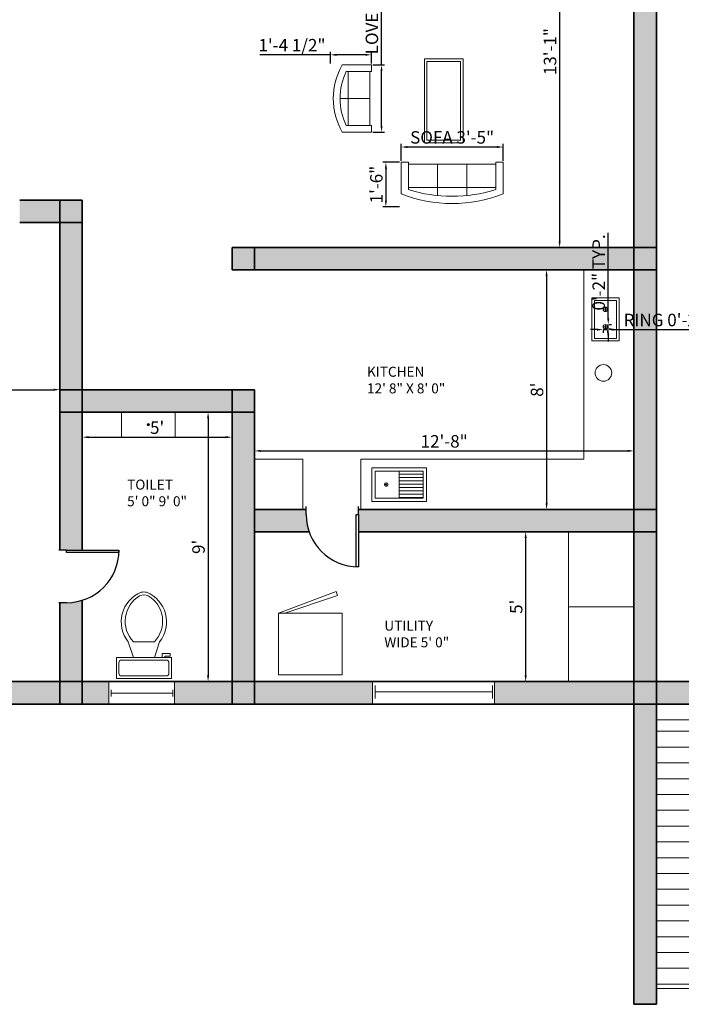
# Model space of a CAD drawing. Units: millimetres. Extents: x 2768 to 4359, y 795 to 1583.
# Tile 2 of 13: x 2961 to 3226, y 891 to 1286. Entities that reach past the tile are written whole.
import ezdxf

# ---------------------------------------------------------------- set-up
doc = ezdxf.new("R2010")
doc.units = ezdxf.units.MM
for name, color, linetype, lineweight in [('A-ANNO-DIMS', 90, 'Continuous', 18), ('A-AREA-IDEN', 190, 'Continuous', 18), ('A-DOOR-PATT', 251, 'Continuous', 13), ('A-EQPM', 50, 'Continuous', 18), ('A-FLOR-CASE', 50, 'Continuous', 18), ('A-FLOR-FIXT', 50, 'Continuous', 18), ('A-FLOR-FIXT-PATT', 50, 'Continuous', 13), ('A-WALL-PATT', 140, 'Continuous', 9), ('doors', 10, 'Continuous', 25), ('furniture', 50, 'Continuous', 18), ('iron shutter', 251, 'Continuous', 18), ('walls', 140, 'Continuous', 35), ('windows', 30, 'Continuous', 18)]:
    doc.layers.add(name, color=color, linetype=linetype, lineweight=lineweight)
doc.styles.get("Standard").update_dxf_attribs({"font": 'arial.ttf'})
doc.dimstyles.new('ISO-25', dxfattribs={"dimtxt": 5, "dimasz": 2.5, "dimexe": 1.25, "dimexo": 0.625, "dimtad": 1, "dimdec": 0, "dimlunit": 3, "dimtxsty": 'Standard', "dimcen": 2.5, "dimadec": 0, "dimazin": 0, "dimtfac": 1, "dimtdec": 0, "dimtmove": 0, "dimatfit": 3, "dimfxl": 1, "dimarcsym": 0})

# ---------------------------------------------------------------- blocks, each defined once
blk = doc.blocks.new('*U2')
for p, q in [((0, 0), (0, -6)), ((40, 0), (40, -6))]:
    blk.add_line(p, q)
blk.add_lwpolyline([(0, 0), (0, 40), (1.75, 40), (1.75, 0)], close=True)
blk.add_arc((0, 0), 40, 0, 90)
blk = doc.blocks.new('*U4')
for p, q in [((0, 4), (0, 0)), ((36, 4), (36, 0)), ((0, 2), (36, 2))]:
    blk.add_line(p, q)
blk = doc.blocks.new('*U5')
for p, q in [((0, 4), (0, 0)), ((0, 2), (36, 2)), ((36, 4), (36, 0))]:
    blk.add_line(p, q)
blk = doc.blocks.new('Toilet - top')
for p, q in [((9.5, -6), (9.5, -2)), ((-10, -8.5), (-8, -8.5)), ((-10, -9.5), (-10, -8.5)), ((-7, -9.5), (-10, -9.5)), ((-8, -8.5), (-8, -8)), ((-7, -8), (-7, -9.5)), ((-4, -8), (-6, -14)), ((4, -8), (6, -14)), ((4, -14), (-4, -14))]:
    blk.add_line(p, q)
blk.add_lwpolyline([(10.5, -8), (10.5, 0), (-10.5, 0), (-10.5, -8)], close=True)
for points in [[(-9.5, -2), (-9.5, -6)], [(8.5, -1), (-8.5, -1)], [(-8.5, -7), (8.5, -7)]]:
    blk.add_lwpolyline(points)
for centre, radius, start, end in [((-8.62, -1.88), 0.884, 81.8699, 188.1301), ((8.62, -1.88), 0.884, 351.8699, 98.1301), ((-8.62, -6.12), 0.884, 171.8699, 278.1301), ((8.62, -6.12), 0.884, 261.8699, 8.1301), ((3.52, -21.58), 12.17, 141.4691, 247.9714), ((4.2, -21.82), 11.33, 136.3677, 238.9468), ((-3.52, -21.58), 12.17, 292.0284, 38.5307), ((-4.2, -21.82), 11.33, 301.053, 43.6321), ((0, -27.88), 4, 245.7318, 294.2682), ((0, -29), 4, 254.8605, 285.1395)]:
    blk.add_arc(centre, radius, start, end)
blk = doc.blocks.new('Sofa - Roundback 7 ft.')
for p, q in [((-12.00002, -32.4421), (-12.00003, -6.5971)), ((11.99997, -32.4421), (11.99998, -6.5971)), ((-36.000027, -34), (-36.000027, -11.4696)), ((-35.999844, -13.3819), (35.9998, -13.3819)), ((35.99998, -34), (35.99998, -11.4696)), ((-36.000027, -32.4421), (35.99998, -32.4421))]:
    blk.add_line(p, q)
for points in [[(-36.000027, -34), (-42.000027, -34), (-42.000027, -8)], [(41.99998, -8), (41.99998, -34), (35.99998, -34)]]:
    blk.add_lwpolyline(points)
for centre, radius, start, end in [((0, -114.25), 114.25, 68.43141, 111.5686), ((-0.00001, -127.1968), 121.1968, 72.72033, 107.2797)]:
    blk.add_arc(centre, radius, start, end)
blk = doc.blocks.new('Sofa - Roundback Loveseat 5 ft.')
for p, q in [((0, -32.44198), (0, -5.99998)), ((-24, -33.99998), (-24, -11.46958)), ((-23.9998, -13.38178), (23.99986, -13.38178)), ((24.00004, -33.99998), (24.00004, -11.46958)), ((-24, -32.44198), (24.00004, -32.44198))]:
    blk.add_line(p, q)
for points in [[(-24, -33.99998), (-30, -33.99998), (-30, -7.99998)], [(30.00004, -7.99998), (30.00004, -33.99998), (24.00004, -33.99998)]]:
    blk.add_lwpolyline(points)
for centre, radius, start, end in [((0, -60.24998), 60.24998, 60.13715, 119.8628), ((0, -61.38438), 55.38444, 64.32083, 115.6792)]:
    blk.add_arc(centre, radius, start, end)
blk = doc.blocks.new('*D22')
at = {"layer": 'A-ANNO-DIMS', "color": 0, "lineweight": -2, "transparency": 16777216}
for p, q in [((2820.41, 1131.43), (2820.41, 1138.66)), ((2822.91, 1137.41), (2974.91, 1137.41)), ((2977.41, 1138.03), (2977.41, 1138.66))]:
    blk.add_line(p, q, dxfattribs=at)
at = {"layer": 'A-ANNO-DIMS', "color": 0, "transparency": 16777216}
for points in [[(2822.91, 1137.82), (2822.91, 1136.99), (2820.41, 1137.41)], [(2974.91, 1137.82), (2974.91, 1136.99), (2977.41, 1137.41)]]:
    blk.add_solid(points, dxfattribs=at)
at = {"layer": 'Defpoints', "color": 0, "transparency": 16777216}
for p in [(2977.41, 1137.41), (2977.41, 1137.41), (2820.41, 1130.8)]:
    blk.add_point(p, dxfattribs=at)
at = {"layer": 'A-ANNO-DIMS', "color": 0, "transparency": 16777216, "insert": (2898.91, 1140.59), "char_height": 5, "attachment_point": 5}
blk.add_mtext('13\'-1"', dxfattribs=at)
blk = doc.blocks.new('*D24')
at = {"layer": 'A-ANNO-DIMS', "color": 0, "lineweight": -2, "transparency": 16777216}
for p, q in [((3041.03, 1128.41), (3035.57, 1128.41)), ((3036.82, 1125.91), (3036.82, 1022.91)), ((3041.03, 1020.41), (3035.57, 1020.41))]:
    blk.add_line(p, q, dxfattribs=at)
at = {"layer": 'A-ANNO-DIMS', "color": 0, "transparency": 16777216}
for points in [[(3036.4, 1125.91), (3037.24, 1125.91), (3036.82, 1128.41)], [(3036.4, 1022.91), (3037.24, 1022.91), (3036.82, 1020.41)]]:
    blk.add_solid(points, dxfattribs=at)
at = {"layer": 'Defpoints', "color": 0, "transparency": 16777216}
for p in [(3041.66, 1128.41), (3036.82, 1020.41), (3041.66, 1020.41)]:
    blk.add_point(p, dxfattribs=at)
at = {"layer": 'A-ANNO-DIMS', "color": 0, "transparency": 16777216, "insert": (3033.64, 1074.41), "char_height": 5, "attachment_point": 5, "rotation": 90}
blk.add_mtext("9'", dxfattribs=at)
blk = doc.blocks.new('*D25')
at = {"layer": 'A-ANNO-DIMS', "color": 0, "lineweight": -2, "transparency": 16777216}
for p, q in [((2986.41, 1121.68), (2986.41, 1117.13)), ((3046.41, 1121.68), (3046.41, 1117.13)), ((2988.91, 1118.38), (3043.91, 1118.38))]:
    blk.add_line(p, q, dxfattribs=at)
at = {"layer": 'A-ANNO-DIMS', "color": 0, "transparency": 16777216}
for points in [[(2988.91, 1118.79), (2988.91, 1117.96), (2986.41, 1118.38)], [(3043.91, 1118.79), (3043.91, 1117.96), (3046.41, 1118.38)]]:
    blk.add_solid(points, dxfattribs=at)
at = {"layer": 'Defpoints', "color": 0, "transparency": 16777216}
for p in [(2986.41, 1122.3), (3046.41, 1122.3), (3046.41, 1118.38)]:
    blk.add_point(p, dxfattribs=at)
at = {"layer": 'A-ANNO-DIMS', "color": 0, "transparency": 16777216, "insert": (3016.41, 1121.54), "char_height": 5, "attachment_point": 5}
blk.add_mtext("5'", dxfattribs=at)
blk = doc.blocks.new('*D26')
at = {"layer": 'A-ANNO-DIMS', "color": 0, "lineweight": -2, "transparency": 16777216}
for p, q in [((3163.77, 1080.41), (3165.3, 1080.41)), ((3164.05, 1077.91), (3164.05, 1022.91)), ((3163.77, 1020.41), (3165.3, 1020.41))]:
    blk.add_line(p, q, dxfattribs=at)
at = {"layer": 'A-ANNO-DIMS', "color": 0, "transparency": 16777216}
for points in [[(3163.63, 1077.91), (3164.47, 1077.91), (3164.05, 1080.41)], [(3163.63, 1022.91), (3164.47, 1022.91), (3164.05, 1020.41)]]:
    blk.add_solid(points, dxfattribs=at)
at = {"layer": 'Defpoints', "color": 0, "transparency": 16777216}
for p in [(3163.14, 1080.41), (3163.14, 1020.41), (3164.05, 1020.41)]:
    blk.add_point(p, dxfattribs=at)
at = {"layer": 'A-ANNO-DIMS', "color": 0, "transparency": 16777216, "insert": (3160.88, 1050.41), "char_height": 5, "attachment_point": 5, "rotation": 90}
blk.add_mtext("5'", dxfattribs=at)
blk = doc.blocks.new('*D27')
at = {"layer": 'A-ANNO-DIMS', "color": 0, "lineweight": -2, "transparency": 16777216}
for p, q in [((3171.15, 1185.41), (3173.68, 1185.41)), ((3172.43, 1182.91), (3172.43, 1091.91)), ((3172.27, 1089.41), (3173.68, 1089.41))]:
    blk.add_line(p, q, dxfattribs=at)
at = {"layer": 'A-ANNO-DIMS', "color": 0, "transparency": 16777216}
for points in [[(3172.01, 1182.91), (3172.85, 1182.91), (3172.43, 1185.41)], [(3172.01, 1091.91), (3172.85, 1091.91), (3172.43, 1089.41)]]:
    blk.add_solid(points, dxfattribs=at)
at = {"layer": 'Defpoints', "color": 0, "transparency": 16777216}
for p in [(3170.52, 1185.41), (3171.64, 1089.41), (3172.43, 1089.41)]:
    blk.add_point(p, dxfattribs=at)
at = {"layer": 'A-ANNO-DIMS', "color": 0, "transparency": 16777216, "insert": (3169.25, 1137.41), "char_height": 5, "attachment_point": 5, "rotation": 90}
blk.add_mtext("8'", dxfattribs=at)
blk = doc.blocks.new('*D28')
at = {"layer": 'A-ANNO-DIMS', "color": 0, "lineweight": -2, "transparency": 16777216}
for p, q in [((3055.41, 1115.69), (3055.41, 1111.63)), ((3057.91, 1112.88), (3204.91, 1112.88)), ((3207.41, 1115.69), (3207.41, 1111.63))]:
    blk.add_line(p, q, dxfattribs=at)
at = {"layer": 'A-ANNO-DIMS', "color": 0, "transparency": 16777216}
for points in [[(3057.91, 1113.3), (3057.91, 1112.46), (3055.41, 1112.88)], [(3204.91, 1113.3), (3204.91, 1112.46), (3207.41, 1112.88)]]:
    blk.add_solid(points, dxfattribs=at)
at = {"layer": 'Defpoints', "color": 0, "transparency": 16777216}
for p in [(3055.41, 1116.31), (3207.41, 1116.31), (3207.41, 1112.88)]:
    blk.add_point(p, dxfattribs=at)
at = {"layer": 'A-ANNO-DIMS', "color": 0, "transparency": 16777216, "insert": (3131.41, 1116.06), "char_height": 5, "attachment_point": 5}
blk.add_mtext('12\'-8"', dxfattribs=at)
blk = doc.blocks.new('*D30')
at = {"layer": 'A-ANNO-DIMS', "color": 0, "lineweight": -2, "transparency": 16777216}
for p, q in [((3177.44, 1351.41), (3178.91, 1351.41)), ((3177.66, 1348.91), (3177.66, 1196.91)), ((3177.44, 1194.41), (3178.91, 1194.41))]:
    blk.add_line(p, q, dxfattribs=at)
at = {"layer": 'A-ANNO-DIMS', "color": 0, "transparency": 16777216}
for points in [[(3177.25, 1348.91), (3178.08, 1348.91), (3177.66, 1351.41)], [(3177.25, 1196.91), (3178.08, 1196.91), (3177.66, 1194.41)]]:
    blk.add_solid(points, dxfattribs=at)
at = {"layer": 'Defpoints', "color": 0, "transparency": 16777216}
for p in [(3176.82, 1351.41), (3176.82, 1194.41), (3177.66, 1194.41)]:
    blk.add_point(p, dxfattribs=at)
at = {"layer": 'A-ANNO-DIMS', "color": 0, "transparency": 16777216, "insert": (3174.48, 1272.91), "char_height": 5, "attachment_point": 5, "rotation": 90}
blk.add_mtext('13\'-1"', dxfattribs=at)
blk = doc.blocks.new('COOKTOP-BURNER')
for p, q in [((1.78, 0.89), (0, 0.89)), ((0.89, 1.78), (0.89, 0))]:
    blk.add_line(p, q)
blk.add_circle((0.89, 0.89), 0.892)
blk = doc.blocks.new('*D103')
at = {"layer": 'A-ANNO-DIMS', "color": 0, "lineweight": -2, "transparency": 16777216}
for p, q in [((3114.17, 1229.16), (3114.17, 1235.91)), ((3155.01, 1229.16), (3155.01, 1235.91)), ((3152.51, 1234.66), (3116.67, 1234.66))]:
    blk.add_line(p, q, dxfattribs=at)
at = {"layer": 'A-ANNO-DIMS', "color": 0, "transparency": 16777216}
for points in [[(3116.67, 1235.08), (3116.67, 1234.24), (3114.17, 1234.66)], [(3152.51, 1235.08), (3152.51, 1234.24), (3155.01, 1234.66)]]:
    blk.add_solid(points, dxfattribs=at)
at = {"layer": 'Defpoints', "color": 0, "transparency": 16777216}
for p in [(3114.17, 1234.66), (3114.17, 1228.53), (3155.01, 1228.53)]:
    blk.add_point(p, dxfattribs=at)
at = {"layer": 'A-ANNO-DIMS', "color": 0, "transparency": 16777216, "insert": (3134.59, 1237.87), "char_height": 5, "attachment_point": 5}
blk.add_mtext('SOFA 3\'-5"', dxfattribs=at)
blk = doc.blocks.new('*D104')
at = {"layer": 'A-ANNO-DIMS', "color": 0, "lineweight": -2, "transparency": 16777216}
for p, q in [((3113.55, 1228.53), (3106.8, 1228.53)), ((3108.05, 1226.03), (3108.05, 1213.21)), ((3113.55, 1210.71), (3106.8, 1210.71))]:
    blk.add_line(p, q, dxfattribs=at)
at = {"layer": 'A-ANNO-DIMS', "color": 0, "transparency": 16777216}
for points in [[(3107.63, 1226.03), (3108.46, 1226.03), (3108.05, 1228.53)], [(3107.63, 1213.21), (3108.46, 1213.21), (3108.05, 1210.71)]]:
    blk.add_solid(points, dxfattribs=at)
at = {"layer": 'Defpoints', "color": 0, "transparency": 16777216}
for p in [(3114.17, 1228.53), (3108.05, 1210.71), (3114.17, 1210.71)]:
    blk.add_point(p, dxfattribs=at)
at = {"layer": 'A-ANNO-DIMS', "color": 0, "transparency": 16777216, "insert": (3104.87, 1219.62), "char_height": 5, "attachment_point": 5, "rotation": 90}
blk.add_mtext('1\'-6"', dxfattribs=at)
blk = doc.blocks.new('*D109')
at = {"layer": 'A-ANNO-DIMS', "color": 0, "lineweight": -2, "transparency": 16777216}
for p, q in [((3106.3, 1267.57), (3106.3, 1323.21)), ((3102.89, 1267.57), (3107.55, 1267.57)), ((3106.3, 1243.13), (3106.3, 1265.07)), ((3102.89, 1240.63), (3107.55, 1240.63))]:
    blk.add_line(p, q, dxfattribs=at)
at = {"layer": 'A-ANNO-DIMS', "color": 0, "transparency": 16777216}
for points in [[(3105.89, 1265.07), (3106.72, 1265.07), (3106.3, 1267.57)], [(3105.89, 1243.13), (3106.72, 1243.13), (3106.3, 1240.63)]]:
    blk.add_solid(points, dxfattribs=at)
at = {"layer": 'Defpoints', "color": 0, "transparency": 16777216}
for p in [(3102.26, 1267.57), (3106.3, 1267.57), (3102.26, 1240.63)]:
    blk.add_point(p, dxfattribs=at)
at = {"layer": 'A-ANNO-DIMS', "color": 0, "transparency": 16777216, "insert": (3103.09, 1296.64), "char_height": 5, "attachment_point": 5, "rotation": 90}
blk.add_mtext('LOVESEAT 2\'-3"', dxfattribs=at)
blk = doc.blocks.new('*D110')
at = {"layer": 'A-ANNO-DIMS', "color": 0, "lineweight": -2, "transparency": 16777216}
for p, q in [((3085.8, 1271.61), (3057.58, 1271.61)), ((3085.8, 1268.19), (3085.8, 1272.86)), ((3099.76, 1271.61), (3088.3, 1271.61)), ((3102.26, 1268.19), (3102.26, 1272.86))]:
    blk.add_line(p, q, dxfattribs=at)
at = {"layer": 'A-ANNO-DIMS', "color": 0, "transparency": 16777216}
for points in [[(3088.3, 1272.03), (3088.3, 1271.19), (3085.8, 1271.61)], [(3099.76, 1272.03), (3099.76, 1271.19), (3102.26, 1271.61)]]:
    blk.add_solid(points, dxfattribs=at)
at = {"layer": 'Defpoints', "color": 0, "transparency": 16777216}
for p in [(3085.8, 1271.61), (3085.8, 1267.57), (3102.26, 1267.57)]:
    blk.add_point(p, dxfattribs=at)
at = {"layer": 'A-ANNO-DIMS', "color": 0, "transparency": 16777216, "insert": (3070.44, 1274.82), "char_height": 5, "attachment_point": 5}
blk.add_mtext('1\'-4 1/2"', dxfattribs=at)
blk = doc.blocks.new('*D121')
at = {"layer": 'A-ANNO-DIMS', "color": 0, "lineweight": -2, "transparency": 16777216}
for p, q in [((3192.58, 1161.48), (3190.08, 1161.48)), ((3195.08, 1161.48), (3196.87, 1161.48)), ((3195.08, 1161.12), (3195.08, 1160.23)), ((3196.87, 1161.12), (3196.87, 1160.23)), ((3199.37, 1161.48), (3252.74, 1161.48))]:
    blk.add_line(p, q, dxfattribs=at)
at = {"layer": 'A-ANNO-DIMS', "color": 0, "transparency": 16777216}
for points in [[(3192.58, 1161.9), (3192.58, 1161.06), (3195.08, 1161.48)], [(3199.37, 1161.9), (3199.37, 1161.06), (3196.87, 1161.48)]]:
    blk.add_solid(points, dxfattribs=at)
at = {"layer": 'Defpoints', "color": 0, "transparency": 16777216}
for p in [(3195.08, 1161.75), (3196.87, 1161.75), (3196.87, 1161.48)]:
    blk.add_point(p, dxfattribs=at)
at = {"layer": 'A-ANNO-DIMS', "color": 0, "transparency": 16777216, "insert": (3227.3, 1164.69), "char_height": 5, "attachment_point": 5}
blk.add_mtext('RING 0\'-2" TYP.', dxfattribs=at)
blk = doc.blocks.new('*D122')
at = {"layer": 'A-ANNO-DIMS', "color": 0, "lineweight": -2, "transparency": 16777216}
for p, q in [((3197.14, 1166.03), (3197.14, 1200.26)), ((3197.14, 1161.75), (3197.14, 1163.53)), ((3197.49, 1163.53), (3198.39, 1163.53)), ((3197.49, 1161.75), (3198.39, 1161.75)), ((3197.14, 1159.25), (3197.14, 1156.75))]:
    blk.add_line(p, q, dxfattribs=at)
at = {"layer": 'A-ANNO-DIMS', "color": 0, "transparency": 16777216}
for points in [[(3196.72, 1166.03), (3197.55, 1166.03), (3197.14, 1163.53)], [(3196.72, 1159.25), (3197.55, 1159.25), (3197.14, 1161.75)]]:
    blk.add_solid(points, dxfattribs=at)
at = {"layer": 'Defpoints', "color": 0, "transparency": 16777216}
for p in [(3196.87, 1163.53), (3196.87, 1161.75), (3197.14, 1163.53)]:
    blk.add_point(p, dxfattribs=at)
at = {"layer": 'A-ANNO-DIMS', "color": 0, "transparency": 16777216, "insert": (3193.96, 1184.4), "char_height": 5, "attachment_point": 5, "rotation": 90}
blk.add_mtext('0\'-2" TYP.', dxfattribs=at)

msp = doc.modelspace()

# ---------------------------------------------------------------- hatches: boundary and pattern name
at = {"layer": 'A-DOOR-PATT'}
h = msp.add_hatch(dxfattribs=at)
h.set_pattern_fill('ANSI31', color=256, scale=1.99444, angle=-45, style=0)
h.paths.add_polyline_path([(3216.41, 1005.07), (3458.41, 1005.07), (3458.41, 897.42), (3216.41, 897.42)])
at = {"layer": 'A-FLOR-FIXT-PATT'}
h = msp.add_hatch(dxfattribs=at)
h.set_pattern_fill('ANSI31', color=256, scale=0.4182515, angle=-45, style=0)
h.paths.add_polyline_path([(3113.39, 1093.91), (3122.99, 1093.91), (3122.99, 1104.82), (3113.39, 1104.82)])
at = {"layer": 'A-WALL-PATT'}
h = msp.add_hatch(color=256, dxfattribs=at)
h.dxf.hatch_style = 1
h.paths.add_polyline_path([(2820.41, 1480.41), (2811.41, 1480.41), (2811.41, 1360.41), (2820.41, 1360.41)])
h.paths.add_polyline_path([(2820.41, 1489.41), (2811.41, 1489.41), (2811.41, 1480.41), (2820.41, 1480.41)])
h.paths.add_polyline_path([(2845.83, 1489.41), (2820.41, 1489.41), (2820.41, 1480.41), (2845.83, 1480.41)])
h.paths.add_polyline_path([(2940.41, 1489.41), (2894.95, 1489.41), (2894.95, 1480.41), (2940.41, 1480.41)])
h.paths.add_polyline_path([(2949.41, 1489.41), (2940.41, 1489.41), (2940.41, 1480.41), (2949.41, 1480.41)])
h.paths.add_polyline_path([(2949.41, 1480.41), (2940.41, 1480.41), (2940.41, 1433.68), (2943.15, 1433.68), (2949.41, 1433.68)])
h.paths.add_polyline_path([(2964.2, 1489.41), (2949.41, 1489.41), (2949.41, 1480.41), (2964.2, 1480.41)])
h.paths.add_polyline_path([(3018.41, 1489.41), (3009.41, 1489.41), (3009.41, 1480.41), (3018.41, 1480.41)])
h.paths.add_polyline_path([(3009.41, 1489.41), (2990.92, 1489.41), (2990.92, 1480.41), (3009.41, 1480.41)])
h.paths.add_polyline_path([(3018.41, 1480.41), (3009.41, 1480.41), (3009.41, 1384.41), (3018.41, 1384.41)])
h.paths.add_polyline_path([(3009.41, 1384.41), (2949.41, 1384.41), (2949.41, 1375.41), (3009.41, 1375.41)])
h.paths.add_polyline_path([(3018.41, 1384.41), (3009.41, 1384.41), (3009.41, 1375.41), (3018.41, 1375.41)])
h.paths.add_polyline_path([(2949.41, 1384.41), (2940.41, 1384.41), (2940.41, 1375.41), (2949.41, 1375.41)])
h.paths.add_polyline_path([(2949.41, 1413.64, -0.075856), (2943.15, 1412.69), (2940.41, 1412.69), (2940.41, 1384.41), (2949.41, 1384.41)])
h.paths.add_polyline_path([(2949.41, 1375.41), (2940.41, 1375.41), (2940.41, 1360.41), (2949.41, 1360.41)])
h.paths.add_polyline_path([(2949.41, 1360.41), (2940.41, 1360.41), (2940.41, 1351.41), (2949.41, 1351.41)])
h.paths.add_polyline_path([(2940.41, 1360.41), (2929.82, 1360.41, -0.054277), (2930.46, 1354.53), (2930.46, 1351.41), (2940.41, 1351.41)])
h.paths.add_polyline_path([(2903.16, 1354.53), (2903.16, 1360.41), (2895.41, 1360.41), (2895.41, 1351.41), (2903.16, 1351.41)])
h.paths.add_polyline_path([(2886.41, 1360.41), (2820.41, 1360.41), (2820.41, 1351.41), (2886.41, 1351.41)])
h.paths.add_polyline_path([(2895.41, 1360.41), (2886.41, 1360.41), (2886.41, 1351.41), (2895.41, 1351.41)])
h.paths.add_polyline_path([(2820.41, 1360.41), (2811.41, 1360.41), (2811.41, 1351.41), (2820.41, 1351.41)])
h.paths.add_polyline_path([(2820.41, 1351.41), (2811.41, 1351.41), (2811.41, 1213.41), (2820.41, 1213.41)])
h.paths.add_polyline_path([(2886.41, 1213.41), (2820.41, 1213.41), (2820.41, 1204.41), (2886.41, 1204.41)])
h.paths.add_polyline_path([(2820.41, 1213.41), (2811.41, 1213.41), (2811.41, 1204.41), (2820.41, 1204.41)])
h.paths.add_polyline_path([(2895.41, 1302), (2886.41, 1302), (2886.41, 1264.47), (2895.41, 1264.47)])
h.paths.add_polyline_path([(2934.05, 1209.82), (2934.05, 1213.41), (2895.41, 1213.41), (2895.41, 1204.41), (2934.59, 1204.41, -0.049949)])
h.paths.add_polyline_path([(2895.41, 1213.41), (2886.41, 1213.41), (2886.41, 1204.41), (2895.41, 1204.41)])
h.paths.add_polyline_path([(3078.41, 1384.41), (3018.41, 1384.41), (3018.41, 1375.41), (3078.41, 1375.41)])
h.paths.add_polyline_path([(3087.41, 1433.68), (3084.62, 1433.68), (3078.41, 1433.68), (3078.41, 1384.41), (3087.41, 1384.41)])
h.paths.add_polyline_path([(3087.41, 1384.41), (3078.41, 1384.41), (3078.41, 1375.41), (3087.41, 1375.41)])
h.paths.add_polyline_path([(3087.41, 1375.41), (3078.41, 1375.41), (3078.41, 1360.41), (3087.41, 1360.41)])
h.paths.add_polyline_path([(3087.41, 1360.41), (3078.41, 1360.41), (3078.41, 1351.41), (3087.41, 1351.41)])
h.paths.add_polyline_path([(3093.5, 1360.41), (3087.41, 1360.41), (3087.41, 1351.41), (3093.5, 1351.41), (3093.5, 1353.18)])
h.paths.add_polyline_path([(3207.41, 1360.41), (3119.82, 1360.41, -0.067042), (3120.8, 1353.18), (3120.8, 1351.41), (3207.41, 1351.41)])
h.paths.add_polyline_path([(3216.41, 1480.41), (3207.41, 1480.41), (3207.41, 1360.41), (3216.41, 1360.41)])
h.paths.add_polyline_path([(3216.41, 1360.41), (3207.41, 1360.41), (3207.41, 1351.41), (3216.41, 1351.41)])
h.paths.add_polyline_path([(3216.41, 1489.41), (3207.41, 1489.41), (3207.41, 1480.41), (3216.41, 1480.41)])
h.paths.add_polyline_path([(3207.41, 1489.41), (3167.11, 1489.41), (3167.11, 1480.41), (3207.41, 1480.41)])
h.paths.add_polyline_path([(3118.27, 1489.41), (3087.41, 1489.41), (3087.41, 1480.41), (3118.27, 1480.41)])
h.paths.add_polyline_path([(3087.41, 1489.41), (3078.41, 1489.41), (3078.41, 1480.41), (3087.41, 1480.41)])
h.paths.add_polyline_path([(3087.41, 1480.41), (3078.41, 1480.41), (3078.41, 1453.72, -0.07525), (3084.62, 1454.66), (3087.41, 1454.66)])
h.paths.add_polyline_path([(3078.41, 1489.41), (3058.65, 1489.41), (3058.65, 1480.41), (3078.41, 1480.41)])
h.paths.add_polyline_path([(3031.86, 1489.41), (3018.41, 1489.41), (3018.41, 1480.41), (3031.86, 1480.41)])
h.paths.add_polyline_path([(3458.41, 1489.41), (3216.41, 1489.41), (3216.41, 1480.41), (3458.41, 1480.41)])
h.paths.add_polyline_path([(3467.41, 1489.41), (3458.41, 1489.41), (3458.41, 1480.41), (3467.41, 1480.41)])
h.paths.add_polyline_path([(3467.41, 1480.41), (3458.41, 1480.41), (3458.41, 1020.41), (3467.41, 1020.41)])
h.paths.add_polyline_path([(3458.41, 1020.41), (3216.41, 1020.41), (3216.41, 1011.41), (3458.41, 1011.41)])
h.paths.add_polyline_path([(3467.41, 1020.41), (3458.41, 1020.41), (3458.41, 1011.41), (3467.41, 1011.41)])
h.paths.add_polyline_path([(3216.41, 1080.41), (3207.41, 1080.41), (3207.41, 1020.41), (3216.41, 1020.41)])
h.paths.add_polyline_path([(3216.41, 1020.41), (3207.41, 1020.41), (3207.41, 1011.41), (3216.41, 1011.41)])
h.paths.add_polyline_path([(3207.41, 1020.41), (3151.59, 1020.41), (3151.59, 1011.41), (3207.41, 1011.41)])
h.paths.add_polyline_path([(3216.41, 1185.41), (3207.41, 1185.41), (3207.41, 1089.41), (3216.41, 1089.41)])
h.paths.add_polyline_path([(3216.41, 1089.41), (3207.41, 1089.41), (3207.41, 1080.41), (3216.41, 1080.41)])
h.paths.add_polyline_path([(3207.41, 1089.41), (3097.07, 1089.41), (3097.07, 1087.42), (3097.07, 1080.41), (3207.41, 1080.41)])
h.paths.add_polyline_path([(3216.41, 1194.41), (3207.41, 1194.41), (3207.41, 1185.41), (3216.41, 1185.41)])
h.paths.add_polyline_path([(3207.41, 1194.41), (3055.41, 1194.41), (3055.41, 1185.41), (3207.41, 1185.41)])
h.paths.add_polyline_path([(3055.41, 1194.41), (3046.41, 1194.41), (3046.41, 1185.41), (3055.41, 1185.41)])
h.paths.add_polyline_path([(3055.41, 1128.41), (3046.41, 1128.41), (3046.41, 1020.41), (3055.41, 1020.41)])
h.paths.add_polyline_path([(3055.41, 1020.41), (3046.41, 1020.41), (3046.41, 1011.41), (3055.41, 1011.41)])
h.paths.add_polyline_path([(3102.66, 1020.41), (3055.41, 1020.41), (3055.41, 1011.41), (3102.66, 1011.41)])
h.paths.add_polyline_path([(3055.41, 1137.41), (3046.41, 1137.41), (3046.41, 1128.41), (3055.41, 1128.41)])
h.paths.add_polyline_path([(3046.41, 1137.41), (2986.41, 1137.41), (2986.41, 1128.41), (3046.41, 1128.41)])
h.paths.add_polyline_path([(2986.41, 1204.41), (2977.41, 1204.41), (2977.41, 1137.41), (2986.41, 1137.41)])
h.paths.add_polyline_path([(2986.41, 1213.41), (2977.41, 1213.41), (2977.41, 1204.41), (2986.41, 1204.41)])
h.paths.add_polyline_path([(2977.41, 1213.41), (2961.35, 1213.41), (2961.35, 1209.82), (2961.35, 1204.41), (2977.41, 1204.41)])
h.paths.add_polyline_path([(2986.41, 1137.41), (2977.41, 1137.41), (2977.41, 1128.41), (2986.41, 1128.41)])
h.paths.add_polyline_path([(2986.41, 1128.41), (2977.41, 1128.41), (2977.41, 1073.04), (2980.14, 1073.04), (2986.41, 1073.04)])
h.paths.add_polyline_path([(2986.41, 1053, -0.075909), (2980.14, 1052.05), (2977.41, 1052.05), (2977.41, 1020.41), (2986.41, 1020.41)])
h.paths.add_polyline_path([(2986.41, 1020.41), (2977.41, 1020.41), (2977.41, 1011.41), (2986.41, 1011.41)])
h.paths.add_polyline_path([(2977.41, 1020.41), (2903.99, 1020.41), (2903.99, 1011.41), (2977.41, 1011.41)])
h.paths.add_polyline_path([(2820.41, 1111.04), (2811.41, 1111.04), (2811.41, 1020.41), (2820.41, 1020.41)])
h.paths.add_polyline_path([(2820.41, 1020.41), (2811.41, 1020.41), (2811.41, 1011.41), (2820.41, 1011.41)])
h.paths.add_polyline_path([(2855.32, 1020.41), (2820.41, 1020.41), (2820.41, 1011.41), (2855.32, 1011.41)])
h.paths.add_polyline_path([(2820.41, 1204.41), (2811.41, 1204.41), (2811.41, 1161.45), (2820.41, 1161.45)])
edge = h.paths.add_edge_path()
edge.add_arc((3211.84, 1295.2), 27.3, 86.9636, 99.352)
edge.add_line((3207.41, 1322.13), (3207.41, 1351.41))
edge.add_line((3207.41, 1351.41), (3216.41, 1351.41))
edge.add_line((3216.41, 1351.41), (3216.41, 1322.29))
edge.add_line((3216.41, 1322.29), (3213.29, 1322.46))
h = msp.add_hatch(color=256, dxfattribs=at)
h.dxf.hatch_style = 1
h.paths.add_polyline_path([(3216.41, 1294.96), (3213.5, 1295.11), (3207.41, 1295.43), (3207.41, 1194.41), (3216.41, 1194.41)])
h.paths.add_polyline_path([(3216.41, 1011.41), (3207.41, 1011.41), (3207.41, 891.09), (3216.41, 891.09)])
h.paths.add_polyline_path([(3467.41, 1011.41), (3458.41, 1011.41), (3458.41, 891.09), (3467.41, 891.09)])
h = msp.add_hatch(color=256, dxfattribs=at)
h.dxf.hatch_style = 1
h.paths.add_polyline_path([(3076.08, 1087.42), (3076.08, 1089.41), (3055.41, 1089.41), (3055.41, 1080.41), (3077.29, 1080.41, -0.085424)])
h = msp.add_hatch(color=256, dxfattribs=at)
h.dxf.hatch_style = 1
h.paths.add_polyline_path([(3046.41, 1020.41), (3023.35, 1020.41), (3023.35, 1011.41), (3046.41, 1011.41)])
h.paths.add_polyline_path([(2997.09, 1020.41), (2986.41, 1020.41), (2986.41, 1011.41), (2997.09, 1011.41)])

# ---------------------------------------------------------------- linework, layer by layer
at = {"layer": 'A-EQPM'}
for p, q in [((3065.07, 1047.82), (3088.07, 1056.59)), ((3088.69, 1054.92), (3067.55, 1047.82)), ((3088.07, 1056.59), (3088.69, 1054.92))]:
    msp.add_line(p, q, dxfattribs=at)
for points in [[(3190.58, 1174.22), (3201.49, 1174.22), (3201.49, 1156.98), (3190.58, 1156.98)], [(3191.58, 1173.22), (3200.49, 1173.22), (3200.49, 1157.98), (3191.58, 1157.98)], [(3065.07, 1047.82), (3090.51, 1047.82), (3090.51, 1023.13), (3065.07, 1023.13)]]:
    msp.add_lwpolyline(points, close=True, dxfattribs=at)
msp.add_circle((3195.21, 1144.13), 3.33, dxfattribs=at)
at = {"layer": 'A-FLOR-CASE'}
for p, q in [((3207.41, 1185.41), (3187.33, 1185.41)), ((3187.33, 1185.41), (3187.33, 1109.56)), ((3074.84, 1109.56), (3055.41, 1109.56)), ((3074.84, 1089.41), (3074.84, 1109.56)), ((3187.33, 1109.56), (3098.04, 1109.56)), ((3098.04, 1089.41), (3098.04, 1109.56)), ((3181.19, 1050.41), (3207.41, 1050.41))]:
    msp.add_line(p, q, dxfattribs=at)
msp.add_lwpolyline([(3207.41, 1080.41), (3181.19, 1080.41), (3181.19, 1020.41), (3207.41, 1020.41)], close=True, dxfattribs=at)
at = {"layer": 'A-FLOR-FIXT'}
msp.add_line((3113.39, 1093.91), (3113.39, 1104.82), dxfattribs=at)
for points in [[(3002.14, 1128.41), (3023.61, 1128.41), (3023.61, 1118.38), (3002.14, 1118.38)], [(3102.45, 1106.15), (3124.32, 1106.15), (3124.32, 1092.58), (3102.45, 1092.58)], [(3103.78, 1104.82), (3122.99, 1104.82), (3122.99, 1093.91), (3103.78, 1093.91)]]:
    msp.add_lwpolyline(points, close=True, dxfattribs=at)
for centre, radius in [((3012.88, 1123.39), 0.507), ((3012.88, 1123.39), 0.165), ((3108.21, 1099.36), 0.739), ((3108.21, 1099.36), 0.261)]:
    msp.add_circle(centre, radius, dxfattribs=at)
at = {"layer": 'furniture'}
for points in [[(3139, 1269.97), (3139, 1236.35), (3123.46, 1236.35), (3123.46, 1269.97)], [(3138, 1268.97), (3138, 1237.35), (3124.46, 1237.35), (3124.46, 1268.97)]]:
    msp.add_lwpolyline(points, close=True, dxfattribs=at)
at = {"layer": 'iron shutter'}
for p, q in [((3216.41, 1005.07), (3458.41, 1005.07)), ((3216.41, 897.42), (3458.41, 897.42))]:
    msp.add_line(p, q, dxfattribs=at)
at = {"layer": 'walls'}
for p, q in [((3207.41, 1295.43), (3207.41, 891.09)), ((3216.41, 1294.96), (3216.41, 891.09)), ((2961.35, 1213.41), (2986.41, 1213.41)), ((2977.41, 1213.41), (2977.41, 1073.04)), ((2986.41, 1213.41), (2986.41, 1073.04)), ((2961.35, 1204.41), (2986.41, 1204.41)), ((3046.41, 1194.41), (3046.41, 1185.41)), ((3046.41, 1194.41), (3216.41, 1194.41)), ((3055.41, 1194.41), (3055.41, 1185.41)), ((3046.41, 1185.41), (3216.41, 1185.41)), ((2977.41, 1137.41), (3055.41, 1137.41)), ((3046.41, 1137.41), (3046.41, 1011.41)), ((3055.41, 1137.41), (3055.41, 1011.41)), ((2977.41, 1128.41), (3055.41, 1128.41)), ((3055.41, 1089.41), (3076.08, 1089.41)), ((3097.07, 1089.41), (3216.41, 1089.41)), ((3055.41, 1080.41), (3077.29, 1080.41)), ((3097.07, 1080.41), (3216.41, 1080.41)), ((2977.41, 1052.05), (2977.41, 1011.41)), ((2986.41, 1053), (2986.41, 1011.41)), ((2811.41, 1020.41), (3055.41, 1020.41)), ((3055.41, 1020.41), (3467.41, 1020.41)), ((2811.41, 1011.41), (3055.41, 1011.41)), ((3055.41, 1011.41), (3467.41, 1011.41)), ((3207.41, 891.09), (3216.41, 891.09))]:
    msp.add_line(p, q, dxfattribs=at)
at = {"layer": 'windows'}
for p, q in [((2997.09, 1020.41), (2997.09, 1011.41)), ((3023.35, 1020.41), (3023.35, 1011.41)), ((3102.66, 1020.41), (3102.66, 1011.41)), ((3151.59, 1020.41), (3151.59, 1011.41))]:
    msp.add_line(p, q, dxfattribs=at)

# ---------------------------------------------------------------- block references
at = {"layer": 'A-EQPM'}
for p in [(3195.09, 1168.73), (3195.09, 1161.75)]:
    msp.add_blockref('COOKTOP-BURNER', p, dxfattribs=at)
at = {"layer": 'A-FLOR-FIXT', "xscale": 1.051204257850905, "yscale": 1.051204257850905, "zscale": 1.051204257850905, "rotation": 180}
msp.add_blockref('Toilet - top', (3011.11, 1021.66), dxfattribs=at)
at = {"layer": 'doors', "xscale": 0.5246855638968122, "yscale": 0.5246855638968122, "zscale": 0.5246855638968122}
for p, rotation in [((3097.07, 1087.42), 180), ((2980.14, 1073.04), 270)]:
    msp.add_blockref('*U2', p, dxfattribs=dict(at, rotation=rotation))
at = {"layer": 'furniture'}
for name, p, xscale, yscale, zscale, rotation in [('Sofa - Roundback Loveseat 5 ft.', (3086.99, 1254.1), 0.4490511546701813, 0.4490511546701813, 0.4490511546701813, 90), ('Sofa - Roundback 7 ft.', (3134.59, 1212), 0.4861771483710998, 0.4861771483710998, 0.4861771483710998, 180)]:
    msp.add_blockref(name, p, dxfattribs=dict(at, xscale=xscale, yscale=yscale, zscale=zscale, rotation=rotation))
at = {"layer": 'windows'}
for name, p, xscale, yscale, zscale in [('*U4', (3103.81, 1013.7), 1.304585616368386, 1.304585616368386, 1.304585616368386), ('*U5', (2998.04, 1014.41), 0.6837569988572593, 0.6837569988572593, 0.6837569988572593)]:
    msp.add_blockref(name, p, dxfattribs=dict(at, xscale=xscale, yscale=yscale, zscale=zscale))

# ---------------------------------------------------------------- texts
at = {"layer": 'A-AREA-IDEN', "char_height": 4, "attachment_point": 1}
for s, width, insert in [('KITCHEN\\P12\' 8" X 8\' 0"', 37.8305, (3100.48, 1146.6)), ('TOILET\\P5\' 0" 9\' 0"', 38.363, (3004.38, 1101.36)), ('UTILITY \\PWIDE 5\' 0"', 32.6359, (3107.43, 1044.84))]:
    msp.add_mtext_dynamic_manual_height_columns(s, width=width, gutter_width=12.5, heights=[0], dxfattribs=dict(at, insert=insert))

# ---------------------------------------------------------------- dimensions: what is measured, and where the dimension line sits
at = {"layer": 'A-ANNO-DIMS'}
for base, p1, p2, angle, override, picture, middle in [((3177.66, 1194.41), (3176.82, 1351.41), (3176.82, 1194.41), 90, {"dimclrd": 0, "dimclre": 0, "dimclrt": 0}, '*D30', (3174.48, 1272.91)), ((3085.8, 1271.61), (3102.26, 1267.57), (3085.8, 1267.57), 180, {"dimdec": 1, "dimlfac": 1, "dimrnd": 0, "dimzin": 1, "dimdsep": 46, "dimlunit": 4, "dimfrac": 2}, '*D110', (3070.44, 1274.82)), ((3108.05, 1210.71), (3114.17, 1228.53), (3114.17, 1210.71), 270, {"dimdec": 1, "dimlfac": 1, "dimrnd": 0, "dimzin": 1, "dimdsep": 46, "dimlunit": 4, "dimfrac": 2}, '*D104', (3104.87, 1219.62)), ((3172.43, 1089.41), (3170.52, 1185.41), (3171.64, 1089.41), 90, {"dimclrd": 0, "dimclre": 0, "dimclrt": 0}, '*D27', (3169.25, 1137.41)), ((3036.82, 1020.41), (3041.66, 1128.41), (3041.66, 1020.41), 90, {"dimclrd": 0, "dimclre": 0, "dimclrt": 0}, '*D24', (3033.64, 1074.41)), ((3164.05, 1020.41), (3163.14, 1080.41), (3163.14, 1020.41), 90, {"dimclrd": 0, "dimclre": 0, "dimclrt": 0}, '*D26', (3160.88, 1050.41))]:
    dim = msp.add_linear_dim(base=base, p1=p1, p2=p2, angle=angle, dimstyle='ISO-25', override=override, dxfattribs=at)
    dim.commit()
    dim.dimension.update_dxf_attribs({"geometry": picture, "text_midpoint": middle})
for base, p1, p2, angle, text, picture, middle in [((3106.3, 1267.57), (3102.26, 1240.63), (3102.26, 1267.57), 90, 'LOVESEAT <>', '*D109', (3103.09, 1296.64)), ((3114.17, 1234.66), (3155.01, 1228.53), (3114.17, 1228.53), 180, 'SOFA <>', '*D103', (3134.59, 1237.87)), ((3197.14, 1163.53), (3196.87, 1161.75), (3196.87, 1163.53), 90, '<> TYP.', '*D122', (3193.96, 1184.4))]:
    dim = msp.add_linear_dim(base=base, p1=p1, p2=p2, angle=angle, text=text, dimstyle='ISO-25', override={"dimdec": 1, "dimlfac": 1, "dimrnd": 0, "dimzin": 1, "dimdsep": 46, "dimlunit": 4, "dimfrac": 2}, dxfattribs=at)
    dim.commit()
    dim.dimension.update_dxf_attribs({"geometry": picture, "text_midpoint": middle})
dim = msp.add_linear_dim(base=(3196.87, 1161.48), p1=(3195.08, 1161.75), p2=(3196.87, 1161.75), text='RING <> TYP.', dimstyle='ISO-25', override={"dimdec": 1, "dimlfac": 1, "dimrnd": 0, "dimzin": 1, "dimdsep": 46, "dimlunit": 4, "dimfrac": 2}, dxfattribs=at)
dim.commit()
dim.dimension.update_dxf_attribs({"geometry": '*D121', "text_midpoint": (3227.3, 1164.69)})
for base, p1, p2, picture, middle in [((2977.41, 1137.41), (2820.41, 1130.8), (2977.41, 1137.41), '*D22', (2898.91, 1140.59)), ((3046.41, 1118.38), (2986.41, 1122.3), (3046.41, 1122.3), '*D25', (3016.41, 1121.54)), ((3207.41, 1112.88), (3055.41, 1116.31), (3207.41, 1116.31), '*D28', (3131.41, 1116.06))]:
    dim = msp.add_linear_dim(base=base, p1=p1, p2=p2, dimstyle='ISO-25', override={"dimclrd": 0, "dimclre": 0, "dimclrt": 0}, dxfattribs=at)
    dim.commit()
    dim.dimension.update_dxf_attribs({"geometry": picture, "text_midpoint": middle})

doc.saveas('drawing.dxf')
